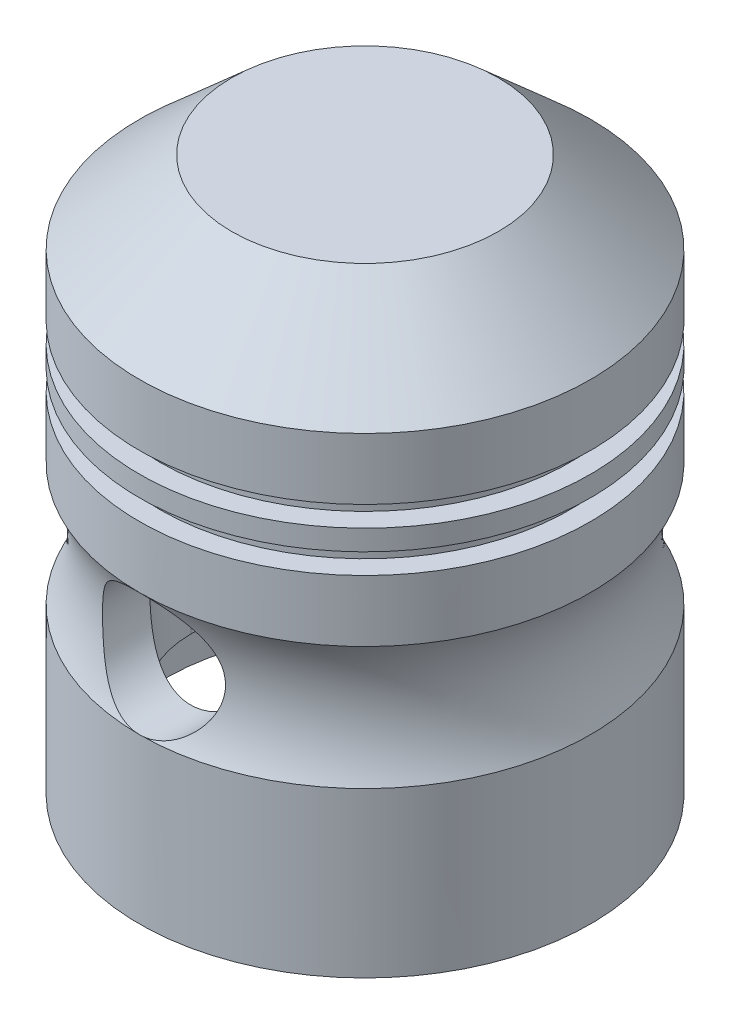
from build123d import *

# Parameters (mm, degrees)
CON_ROD_SLOT_DEPTH        = 19
UNDERSIDE_BORE_SKETCH_R   = 9.75
UNDERSIDE_BORE_19_5_DEPTH = 6
WRIST_PIN_HOLE_SKETCH_R   = 3
WRIST_PIN_HOLE_6_DEPTH    = 18.500000000000004


with BuildPart() as part:
    # Piston Profile Sketch → Piston Body (revolve)
    with BuildSketch(Plane.XY, mode=Mode.PRIVATE) as piston_body_sk:
        with BuildLine():
            Line((0, -12.6437125748503), (11.000000000000002, -12.6437125748503))
            Line((11.000000000000002, -12.6437125748503), (11.000000000000002, -4.643712574850299))
            ThreePointArc((11.000000000000002, -4.643712574850299), (10.250666035204008, -1.6437125748502983), (11.000000000000002, 1.3562874251497004))
            Line((11.000000000000002, 1.3562874251497004), (11.000000000000002, 4.356287425149702))
            Line((11.000000000000002, 4.356287425149702), (10.000000000000002, 4.356287425149703))
            Line((10.000000000000002, 4.356287425149703), (10.000000000000002, 5.3562874251496995))
            Line((10.000000000000002, 5.3562874251496995), (11, 5.3562874251496995))
            Line((11, 5.3562874251496995), (11, 6.3562874251497))
            Line((11, 6.3562874251497), (10.000000000000002, 6.356287425149702))
            Line((10.000000000000002, 6.356287425149702), (10.000000000000002, 7.356287425149701))
            Line((10.000000000000002, 7.356287425149701), (11.000000000000002, 7.356287425149701))
            Line((11.000000000000002, 7.356287425149701), (11.000000000000002, 10.356287425149699))
            Line((11.000000000000002, 10.356287425149699), (6.5, 14.356287425149699))
            Line((6.5, 14.356287425149699), (-1.8e-16, 14.356287425149699))
            Line((-1.8e-16, 14.356287425149699), (0, -12.6437125748503))
        make_face()
    revolve(piston_body_sk.sketch.rotate(Axis((0, -15.6437125748503, 0), (0, 1, 0)), 90), axis=Axis((0, -15.6437125748503, 0), (0, 1, 0)))

    # Con Rod Slot Sketch → Con Rod Slot (cut)
    with BuildSketch(Plane.XZ.offset(12.6437125748503)):
        with BuildLine():
            Line((-4.999999999999999, -3.5000000000000013), (-5.000000000000002, 3.499999999999997))
            ThreePointArc((-5.000000000000002, 3.499999999999997), (-3.54e-15, 8.500000000000002), (5, 3.500000000000003))
            Line((5, 3.500000000000003), (5.000000000000003, -3.4999999999999987))
            ThreePointArc((5.000000000000003, -3.4999999999999987), (2.79e-15, -8.5), (-4.999999999999999, -3.5000000000000013))
        make_face()
    extrude(amount=-CON_ROD_SLOT_DEPTH, mode=Mode.SUBTRACT)

    # Underside Bore Sketch → Underside Bore Ø19.5 (cut)
    with BuildSketch(Plane.XZ.offset(12.6437125748503)):
        with Locations(Location((0, 0, 0), (0, 0, 270))):
            Circle(UNDERSIDE_BORE_SKETCH_R)
    extrude(amount=-UNDERSIDE_BORE_19_5_DEPTH, mode=Mode.SUBTRACT)

    # Wrist Pin Hole Sketch → Wrist Pin Hole Ø6 (cut, symmetric)
    with BuildSketch(Plane.XY):
        with Locations((0, -1.6437125748502988)):
            Circle(WRIST_PIN_HOLE_SKETCH_R)
    extrude(amount=WRIST_PIN_HOLE_6_DEPTH, both=True, mode=Mode.SUBTRACT)


solid = part.part
